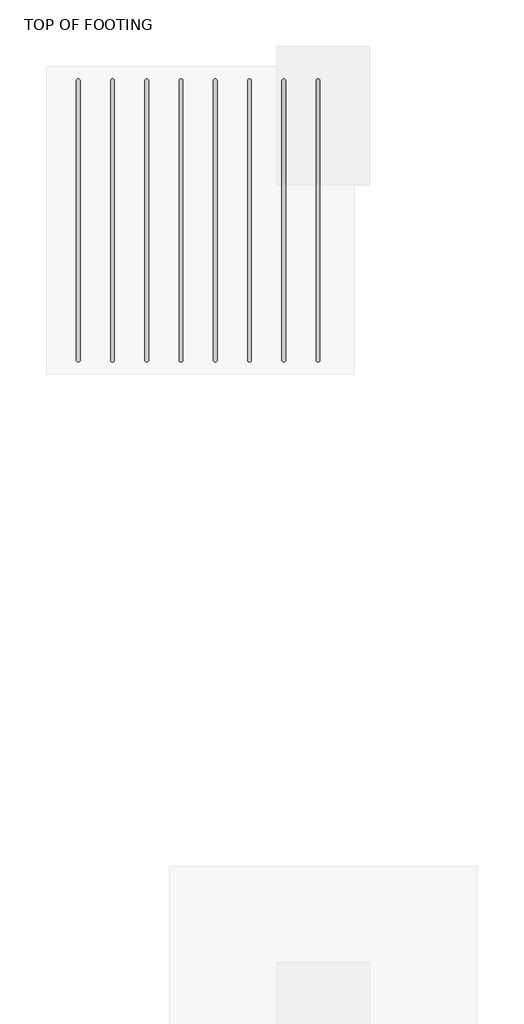
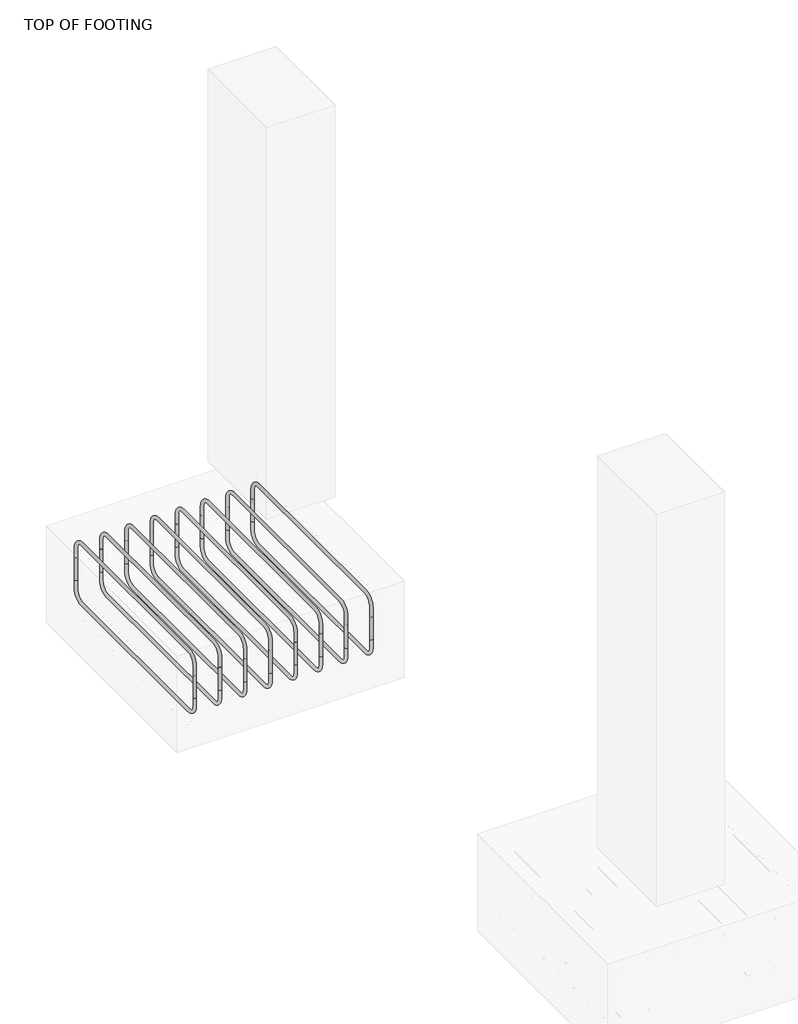
# One storey, part 20 of 20: 2 reinforcing bars.
"""IFC4 building model written with IfcOpenShell, lengths in millimetres."""

from ifc_helpers import new_model, si_unit, point, frame, origin, place, context, project, spatial, polyline, circle_curve, trimmed, segment, composite_curve, source, transform, mapped, element, save
from ifc_brep_helpers import swept_disk

model = new_model("IFC4")

# Units and contexts
model_context = context("Model", 3, world=origin())
ifc_project = project(units=[si_unit("LENGTHUNIT", "METRE", prefix="MILLI")], contexts=[model_context])

# Site, building, storey
site = spatial("IfcSite", under=ifc_project)
building = spatial("IfcBuilding", under=site)
storey = spatial("IfcBuildingStorey", under=building, Name="TOP OF FOOTING", Elevation=-1828.8)

# Reinforcing bars
placement = place(None, origin())
reinforcing_bar_shape = source(origin(), model_context, "Body", "SolidModel", [
    swept_disk(composite_curve([segment(polyline([(12751.2694294, 21841.4849362, -2086.1951968), (12751.2694294, 21841.4849362, -1938.8951968)]), True, "CONTINUOUS"), segment(trimmed(circle_curve(frame((12751.2694294, 21795.1349362, -1938.8951968), z_axis=(1.0, 0.0, 0.0), x_axis=(0.0, 46.349999999998545, 0.0)), 46.35), [point((12751.2694294, 21841.4849362, -1938.8951968))], [point((12751.2694294, 21795.1349362, -1892.5451968))], True, "CARTESIAN"), True, "CONTINUOUS"), segment(polyline([(12751.2694294, 21795.1349362, -1892.5451968), (12751.2694294, 20980.5349362, -1892.5451968)]), True, "CONTINUOUS"), segment(trimmed(circle_curve(frame((12751.2694294, 20980.5349362, -1938.8951968), z_axis=(1.0, 0.0, 0.0), x_axis=(0.0, 0.0, 46.34999999999991)), 46.35), [point((12751.2694294, 20980.5349362, -1892.5451968))], [point((12751.2694294, 20934.1849362, -1938.8951968))], True, "CARTESIAN"), True, "CONTINUOUS"), segment(polyline([(12751.2694294, 20934.1849362, -1938.8951968), (12751.2694294, 20934.1849362, -2086.1951968)]), True, "CONTINUOUS")], self_intersect=False), 6.35),
])
element("IfcReinforcingBar", 1, at=placement, inside=storey, context=model_context, shape_type="MappedRepresentation", body=[
    mapped(reinforcing_bar_shape, transform((0.0, 0.0, 0.0), x_axis=(1.0, 0.0, 0.0), y_axis=(0.0, 1.0, 0.0), z_axis=(0.0, 0.0, 1.0))),
    mapped(reinforcing_bar_shape, transform((-111.2862402, 0.0, 0.0), x_axis=(1.0, 0.0, 0.0), y_axis=(0.0, 1.0, 0.0), z_axis=(0.0, 0.0, 1.0))),
    mapped(reinforcing_bar_shape, transform((-222.5724804, 0.0, 0.0), x_axis=(1.0, 0.0, 0.0), y_axis=(0.0, 1.0, 0.0), z_axis=(0.0, 0.0, 1.0))),
    mapped(reinforcing_bar_shape, transform((-333.8587205, 0.0, 0.0), x_axis=(1.0, 0.0, 0.0), y_axis=(0.0, 1.0, 0.0), z_axis=(0.0, 0.0, 1.0))),
    mapped(reinforcing_bar_shape, transform((-445.1449607, 0.0, 0.0), x_axis=(1.0, 0.0, 0.0), y_axis=(0.0, 1.0, 0.0), z_axis=(0.0, 0.0, 1.0))),
    mapped(reinforcing_bar_shape, transform((-556.4312009, 0.0, 0.0), x_axis=(1.0, 0.0, 0.0), y_axis=(0.0, 1.0, 0.0), z_axis=(0.0, 0.0, 1.0))),
    mapped(reinforcing_bar_shape, transform((-667.7174411, 0.0, 0.0), x_axis=(1.0, 0.0, 0.0), y_axis=(0.0, 1.0, 0.0), z_axis=(0.0, 0.0, 1.0))),
    mapped(reinforcing_bar_shape, transform((-779.0036813, 0.0, 0.0), x_axis=(1.0, 0.0, 0.0), y_axis=(0.0, 1.0, 0.0), z_axis=(0.0, 0.0, 1.0))),
])
reinforcing_bar_2_shape = source(origin(), model_context, "Body", "SolidModel", [
    swept_disk(composite_curve([segment(polyline([(11972.2657481, 21841.4849362, -1979.1645013), (11972.2657481, 21841.4849362, -2126.4645013)]), True, "CONTINUOUS"), segment(trimmed(circle_curve(frame((11972.2657481, 21795.1349362, -2126.4645013), z_axis=(-1.0, 0.0, 0.0), x_axis=(0.0, 46.349999999998545, 0.0)), 46.35), [point((11972.2657481, 21841.4849362, -2126.4645013))], [point((11972.2657481, 21795.1349362, -2172.8145013))], True, "CARTESIAN"), True, "CONTINUOUS"), segment(polyline([(11972.2657481, 21795.1349362, -2172.8145013), (11972.2657481, 20980.5349362, -2172.8145013)]), True, "CONTINUOUS"), segment(trimmed(circle_curve(frame((11972.2657481, 20980.5349362, -2126.4645013), z_axis=(-1.0, 0.0, 0.0), x_axis=(0.0, 0.0, -46.34999999999991)), 46.35), [point((11972.2657481, 20980.5349362, -2172.8145013))], [point((11972.2657481, 20934.1849362, -2126.4645013))], True, "CARTESIAN"), True, "CONTINUOUS"), segment(polyline([(11972.2657481, 20934.1849362, -2126.4645013), (11972.2657481, 20934.1849362, -1979.1645013)]), True, "CONTINUOUS")], self_intersect=False), 6.35),
])
element("IfcReinforcingBar", 2, at=placement, inside=storey, context=model_context, shape_type="MappedRepresentation", body=[
    mapped(reinforcing_bar_2_shape, transform((0.0, 0.0, 0.0), x_axis=(1.0, 0.0, 0.0), y_axis=(0.0, 1.0, 0.0), z_axis=(0.0, 0.0, 1.0))),
    mapped(reinforcing_bar_2_shape, transform((111.2862402, 0.0, 0.0), x_axis=(1.0, 0.0, 0.0), y_axis=(0.0, 1.0, 0.0), z_axis=(0.0, 0.0, 1.0))),
    mapped(reinforcing_bar_2_shape, transform((222.5724804, 0.0, 0.0), x_axis=(1.0, 0.0, 0.0), y_axis=(0.0, 1.0, 0.0), z_axis=(0.0, 0.0, 1.0))),
    mapped(reinforcing_bar_2_shape, transform((333.8587205, 0.0, 0.0), x_axis=(1.0, 0.0, 0.0), y_axis=(0.0, 1.0, 0.0), z_axis=(0.0, 0.0, 1.0))),
    mapped(reinforcing_bar_2_shape, transform((445.1449607, 0.0, 0.0), x_axis=(1.0, 0.0, 0.0), y_axis=(0.0, 1.0, 0.0), z_axis=(0.0, 0.0, 1.0))),
    mapped(reinforcing_bar_2_shape, transform((556.4312009, 0.0, 0.0), x_axis=(1.0, 0.0, 0.0), y_axis=(0.0, 1.0, 0.0), z_axis=(0.0, 0.0, 1.0))),
    mapped(reinforcing_bar_2_shape, transform((667.7174411, 0.0, 0.0), x_axis=(1.0, 0.0, 0.0), y_axis=(0.0, 1.0, 0.0), z_axis=(0.0, 0.0, 1.0))),
    mapped(reinforcing_bar_2_shape, transform((779.0036813, 0.0, 0.0), x_axis=(1.0, 0.0, 0.0), y_axis=(0.0, 1.0, 0.0), z_axis=(0.0, 0.0, 1.0))),
])

save(model, "model.ifc")

# Revit data of these elements
# Elements 1, 2 (IfcReinforcingBar)
#   Phase Created = New Construction
